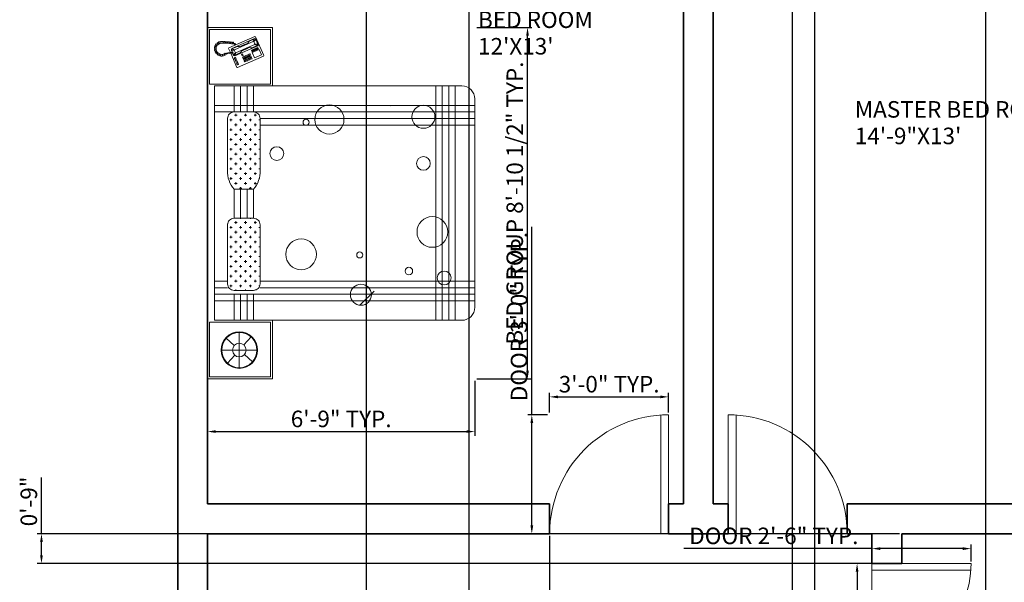
# Model space of a CAD drawing. Units: inches. Extents: x 1265 to 2734, y 1741 to 2595.
# Tile 8 of 10: x 2281 to 2579, y 2294 to 2464. Entities that reach past the tile are written whole.
import ezdxf

# ---------------------------------------------------------------- set-up
doc = ezdxf.new("R2010")
doc.units = ezdxf.units.IN
doc.header["$LTSCALE"] = 0.1
for name, color, linetype, lineweight in [('A-ANNO-DIMS', 2, 'Continuous', 18), ('A-AREA-IDEN', 7, 'Continuous', 18), ('A-DOOR', 3, 'Continuous', 18), ('A-WALL', 7, 'Continuous', 35), ('C-PROP', 7, 'Continuous', 35), ('Furniture', 8, 'Continuous', 15)]:
    doc.layers.add(name, color=color, linetype=linetype, lineweight=lineweight)
doc.styles.get("Standard").update_dxf_attribs({"font": 'arial.ttf', "height": 5})
doc.dimstyles.new('ISO-25', dxfattribs={"dimtxt": 5, "dimasz": 2.5, "dimexe": 1.25, "dimexo": 0.625, "dimtad": 1, "dimlunit": 3, "dimtxsty": 'Standard', "dimcen": 2.5, "dimadec": 0, "dimazin": 0, "dimtfac": 1, "dimtmove": 0, "dimatfit": 3, "dimfxl": 1, "dimarcsym": 0})

# ---------------------------------------------------------------- blocks, each defined once
blk = doc.blocks.new('DOOR-SWING-30IN')
for p, q in [((30, 0), (30, 30)), ((0.07, 2), (30, 2)), ((0, 0), (30, 0))]:
    blk.add_line(p, q)
blk.add_arc((30, 0), 30, 90, 180)
blk = doc.blocks.new('DOOR-SWING-36IN')
for p, q in [((33.6, 35.92), (33.6, 0)), ((36, 36), (36, 0)), ((36, 0), (0, 0))]:
    blk.add_line(p, q)
blk.add_arc((36, 0), 36, 90, 180)
blk = doc.blocks.new('BED-DOUBLE-WITH-NIGHTSTANDS')
h = blk.add_hatch()
h.set_pattern_fill('CROSS', color=256, scale=5.9055, angle=450, style=0)
h.set_pattern_definition([(90, (-724.7185, -618.2252), (1.476375, 1.476375), [0.7381875, -2.2145625]), (360, (-725.0876, -617.8561), (1.476375, -1.476375), [0.7381875, -2.2145625])])
h.paths.add_polyline_path([(13.93, 48.57), (8.02, 48.57, 0.414214), (6.06, 46.6), (6.06, 28.74, 0.414214), (8.02, 26.77), (13.93, 26.77, 0.414214), (15.9, 28.74), (15.9, 46.6, 0.414214)])
h.paths.add_polyline_path([(6.06, 62.99, 0.19223), (8.02, 57.33), (13.93, 57.33, 0.19223), (15.9, 62.99), (15.9, 78.74, 0.414214), (13.93, 80.71), (8.02, 80.71, 0.414214), (6.06, 78.74)])
for p, q in [((0, 0), (0, 106.3)), ((19.69, 106.3), (0, 106.3)), ((19.09, 105.71), (0.59, 105.71)), ((0.59, 105.71), (0.59, 89.17)), ((19.09, 105.71), (19.09, 89.17)), ((19.69, 106.3), (19.69, 88.58)), ((2.44, 101.15), (2.63, 101.34)), ((2.63, 101.34), (3.06, 101.2)), ((2.89, 101.55), (3.11, 101.7)), ((3.06, 101.2), (2.89, 101.55)), ((3.69, 101.46), (2.9, 100.92)), ((3.11, 101.7), (3.41, 101.48)), ((3.36, 101.88), (3.67, 101.95)), ((3.41, 101.48), (3.36, 101.88)), ((3.67, 101.95), (3.81, 101.64)), ((4.95, 101.56), (3.69, 101.46)), ((3.81, 101.64), (3.94, 101.98)), ((3.94, 101.98), (4.24, 102.02)), ((4.24, 102.02), (4.39, 101.64)), ((4.37, 102.03), (4.76, 102.08)), ((4.39, 101.64), (4.37, 102.03)), ((4.76, 102.08), (4.88, 101.72)), ((4.88, 101.72), (5.13, 102.07)), ((5.79, 101.48), (4.95, 101.56)), ((5.13, 102.07), (5.37, 102.03)), ((5.37, 102.03), (5.42, 101.66)), ((5.42, 101.66), (5.65, 101.97)), ((5.65, 101.97), (5.95, 101.95)), ((5.86, 101.55), (5.79, 101.48)), ((5.92, 101.48), (5.86, 101.55)), ((6.5, 101.45), (5.92, 101.48)), ((5.95, 101.95), (5.98, 101.59)), ((5.98, 101.59), (6.16, 101.92)), ((6.16, 101.92), (6.47, 101.91)), ((14.35, 103.55), (6.45, 100.09)), ((6.47, 101.91), (6.46, 101.54)), ((6.46, 101.54), (6.62, 101.9)), ((7.29, 101.35), (6.5, 101.45)), ((6.62, 101.9), (6.85, 101.89)), ((6.85, 101.89), (6.89, 101.51)), ((6.89, 101.51), (7.15, 101.84)), ((7.15, 101.84), (7.36, 101.82)), ((7.73, 101.29), (7.29, 101.35)), ((14.21, 102.94), (7.34, 99.94)), ((7.36, 101.82), (7.4, 101.48)), ((7.4, 101.48), (7.62, 101.8)), ((7.62, 101.8), (7.77, 101.81)), ((7.79, 101.48), (7.73, 101.29)), ((7.77, 101.81), (7.86, 101.7)), ((7.84, 101.37), (7.79, 101.48)), ((7.94, 101.33), (7.84, 101.37)), ((7.86, 101.7), (7.96, 101.49)), ((8.11, 101.22), (7.94, 101.33)), ((7.96, 101.49), (8.25, 101.43)), ((8.25, 101.43), (8.4, 101.32)), ((8.4, 101.32), (8.57, 101.02)), ((11.78, 101.33), (11.2, 101.08)), ((11.28, 100.91), (13.85, 102.03)), ((12.15, 101.56), (11.78, 101.33)), ((12.36, 101.86), (12.15, 101.56)), ((12.6, 102.1), (12.36, 101.86)), ((14.14, 102.78), (12.6, 102.1)), ((14.14, 102.78), (13.85, 102.03)), ((13.85, 102.03), (13.99, 102.03)), ((13.99, 102.03), (14.61, 102.64)), ((13.99, 102.03), (14.34, 101.23)), ((14.4, 102.82), (14.14, 102.78)), ((14.62, 102.78), (14.21, 102.94)), ((14.52, 103.48), (14.35, 103.55)), ((14.61, 102.64), (14.4, 102.82)), ((17.02, 97.76), (14.52, 103.48)), ((15.21, 101.26), (14.61, 102.64)), ((15.37, 101.06), (14.62, 102.78)), ((2.06, 100.15), (2.14, 100.41)), ((2.46, 100.04), (2.06, 100.15)), ((2.09, 99.7), (2.1, 99.92)), ((2.44, 99.53), (2.09, 99.7)), ((2.1, 99.92), (2.46, 100.04)), ((2.13, 99.38), (2.44, 99.53)), ((2.17, 99.14), (2.13, 99.38)), ((2.14, 100.41), (2.51, 100.41)), ((2.59, 99.17), (2.17, 99.14)), ((2.23, 100.67), (2.3, 100.88)), ((2.51, 100.41), (2.23, 100.67)), ((2.29, 98.95), (2.59, 99.17)), ((2.4, 98.76), (2.29, 98.95)), ((2.3, 100.88), (2.69, 100.86)), ((2.78, 98.76), (2.4, 98.76)), ((2.69, 100.86), (2.44, 101.15)), ((2.53, 98.47), (2.78, 98.76)), ((2.71, 98.26), (2.53, 98.47)), ((2.9, 100.92), (2.62, 100.19)), ((2.62, 100.19), (2.62, 99.39)), ((2.62, 99.39), (2.99, 98.72)), ((3.07, 98.46), (2.71, 98.26)), ((2.96, 98.08), (3.07, 98.46)), ((2.99, 98.72), (3.58, 98.25)), ((4.33, 98.05), (5.08, 98.31)), ((5.08, 98.31), (5.33, 98.48)), ((5.33, 98.48), (5.57, 98.34)), ((5.57, 98.34), (5.87, 98.48)), ((5.98, 98.32), (5.68, 98.18)), ((5.87, 98.48), (6.16, 98.57)), ((6.58, 98.42), (5.98, 98.32)), ((6.16, 98.57), (6.77, 98.66)), ((6.45, 100.09), (6.38, 99.93)), ((6.38, 99.93), (6.92, 98.7)), ((7.23, 98.53), (6.58, 98.42)), ((6.77, 98.66), (7.17, 98.75)), ((7.01, 98.5), (8.89, 94.2)), ((7.34, 99.94), (7.12, 99.5)), ((7.12, 99.5), (7.41, 98.83)), ((7.17, 98.75), (7.65, 98.91)), ((7.23, 99.41), (7.24, 99.69)), ((8.1, 99.45), (7.23, 99.41)), ((7.47, 98.85), (7.23, 99.41)), ((7.72, 98.74), (7.23, 98.53)), ((7.24, 99.69), (7.44, 99.85)), ((7.44, 99.85), (8.99, 100.52)), ((7.44, 99.85), (8.18, 99.56)), ((7.49, 98.64), (7.84, 97.84)), ((7.83, 98.04), (7.55, 98.67)), ((7.65, 98.91), (7.72, 98.74)), ((8.45, 98.65), (7.83, 98.04)), ((8.18, 99.56), (8.1, 99.45)), ((8.1, 99.45), (8.45, 98.65)), ((8.26, 101.14), (8.11, 101.22)), ((11.28, 100.91), (8.18, 99.56)), ((8.4, 100.95), (8.26, 101.14)), ((8.26, 97.68), (15.19, 100.71)), ((8.3, 97.9), (8.59, 98.64)), ((8.3, 97.9), (9.84, 98.58)), ((8.59, 98.64), (8.45, 98.65)), ((11.68, 99.99), (8.59, 98.64)), ((8.99, 100.52), (9.33, 100.53)), ((9.33, 100.53), (9.69, 100.49)), ((9.69, 100.49), (10.11, 100.6)), ((9.84, 98.58), (10.08, 98.82)), ((10.08, 98.82), (10.29, 99.11)), ((10.11, 100.6), (11.2, 101.08)), ((10.29, 99.11), (10.66, 99.34)), ((10.66, 99.34), (11.75, 99.82)), ((11.68, 99.99), (14.26, 101.12)), ((12.33, 100.07), (11.75, 99.82)), ((12.75, 100.19), (12.33, 100.07)), ((12.82, 98.31), (12.48, 98.16)), ((13.11, 100.14), (12.75, 100.19)), ((12.97, 97.97), (12.82, 98.31)), ((13.45, 100.15), (13.11, 100.14)), ((13.3, 99.4), (13.47, 99.48)), ((13.5, 98.95), (13.3, 99.4)), ((15, 100.83), (13.45, 100.15)), ((15.58, 99.65), (13.46, 98.72)), ((13.46, 98.72), (14.19, 97.06)), ((13.47, 99.48), (13.67, 99.02)), ((13.67, 99.02), (13.5, 98.95)), ((13.64, 99.55), (13.81, 99.63)), ((13.84, 99.1), (13.64, 99.55)), ((13.81, 99.63), (14.01, 99.17)), ((14.01, 99.17), (13.84, 99.1)), ((13.99, 99.7), (14.16, 99.78)), ((14.19, 99.25), (13.99, 99.7)), ((14.16, 99.78), (14.36, 99.32)), ((14.36, 99.32), (14.19, 99.25)), ((14.26, 101.12), (14.34, 101.23)), ((15, 100.83), (14.26, 101.12)), ((14.33, 99.85), (14.5, 99.93)), ((14.53, 99.4), (14.33, 99.85)), ((14.34, 101.23), (15.21, 101.26)), ((14.5, 99.93), (14.7, 99.47)), ((14.7, 99.47), (14.53, 99.4)), ((14.67, 100), (14.85, 100.08)), ((14.87, 99.55), (14.67, 100)), ((14.85, 100.08), (15.05, 99.62)), ((15.05, 99.62), (14.87, 99.55)), ((15.2, 100.99), (15, 100.83)), ((15.02, 100.16), (15.19, 100.23)), ((15.22, 99.7), (15.02, 100.16)), ((15.19, 100.71), (15.37, 101.06)), ((15.19, 100.23), (15.39, 99.77)), ((15.21, 101.26), (15.2, 100.99)), ((15.39, 99.77), (15.22, 99.7)), ((16.3, 97.99), (15.58, 99.65)), ((3.2, 97.92), (2.96, 98.08)), ((3.49, 98.1), (3.2, 97.92)), ((3.41, 97.75), (3.49, 98.1)), ((3.7, 97.67), (3.41, 97.75)), ((3.58, 98.25), (4.33, 98.05)), ((3.95, 97.97), (3.7, 97.67)), ((4.03, 97.59), (3.95, 97.97)), ((4.36, 97.56), (4.03, 97.59)), ((4.48, 97.99), (4.36, 97.56)), ((4.67, 97.64), (4.48, 97.99)), ((5, 97.75), (4.67, 97.64)), ((5.05, 98.16), (5, 97.75)), ((5.26, 97.85), (5.05, 98.16)), ((5.53, 98), (5.26, 97.85)), ((5.6, 98.18), (5.53, 98)), ((5.68, 98.18), (5.6, 98.18)), ((7.83, 98.04), (8.04, 97.86)), ((7.84, 97.84), (8.26, 97.68)), ((8.04, 97.86), (8.3, 97.9)), ((8.09, 97.13), (8.43, 97.28)), ((8.34, 96.55), (8.09, 97.13)), ((8.68, 96.7), (8.34, 96.55)), ((8.43, 97.28), (8.68, 96.7)), ((8.44, 96.33), (8.78, 96.48)), ((8.69, 95.75), (8.44, 96.33)), ((9.03, 95.9), (8.69, 95.75)), ((8.78, 96.48), (9.03, 95.9)), ((8.79, 95.52), (9.13, 95.67)), ((9.04, 94.95), (8.79, 95.52)), ((9.05, 94.14), (16.96, 97.59)), ((9.13, 95.67), (9.38, 95.1)), ((10.58, 98.29), (10.24, 98.14)), ((10.24, 98.14), (10.44, 97.68)), ((10.44, 97.68), (10.78, 97.83)), ((10.78, 97.83), (10.58, 98.29)), ((10.93, 97.48), (10.59, 97.33)), ((10.59, 97.33), (10.74, 96.99)), ((10.74, 96.99), (11.08, 97.14)), ((11.18, 96.91), (10.84, 96.76)), ((10.84, 96.76), (10.99, 96.42)), ((11.08, 97.14), (10.93, 97.48)), ((10.99, 96.42), (11.33, 96.57)), ((11.43, 96.34), (11.09, 96.19)), ((11.09, 96.19), (11.24, 95.84)), ((11.33, 96.57), (11.18, 96.91)), ((11.56, 97.76), (11.22, 97.61)), ((11.22, 97.61), (11.37, 97.26)), ((11.24, 95.84), (11.58, 95.99)), ((11.37, 97.26), (11.71, 97.42)), ((11.58, 95.99), (11.43, 96.34)), ((11.81, 97.19), (11.47, 97.04)), ((11.47, 97.04), (11.62, 96.69)), ((11.71, 97.42), (11.56, 97.76)), ((11.62, 96.69), (11.96, 96.84)), ((12.06, 96.61), (11.72, 96.46)), ((11.72, 96.46), (11.87, 96.12)), ((11.96, 96.84), (11.81, 97.19)), ((12.19, 98.03), (11.85, 97.88)), ((11.85, 97.88), (12, 97.54)), ((11.87, 96.12), (12.21, 96.27)), ((12, 97.54), (12.34, 97.69)), ((12.21, 96.27), (12.06, 96.61)), ((12.44, 97.46), (12.1, 97.31)), ((12.1, 97.31), (12.25, 96.97)), ((12.34, 97.69), (12.19, 98.03)), ((12.25, 96.97), (12.59, 97.12)), ((12.69, 96.89), (12.35, 96.74)), ((12.35, 96.74), (12.5, 96.39)), ((12.59, 97.12), (12.44, 97.46)), ((12.48, 98.16), (12.63, 97.82)), ((12.5, 96.39), (12.84, 96.55)), ((12.63, 97.82), (12.97, 97.97)), ((12.84, 96.55), (12.69, 96.89)), ((13.07, 97.74), (12.73, 97.59)), ((12.73, 97.59), (12.88, 97.24)), ((12.88, 97.24), (13.22, 97.39)), ((13.32, 97.16), (12.98, 97.01)), ((12.98, 97.01), (13.13, 96.67)), ((13.22, 97.39), (13.07, 97.74)), ((13.13, 96.67), (13.47, 96.82)), ((13.47, 96.82), (13.32, 97.16)), ((14.19, 97.06), (16.3, 97.99)), ((16.96, 97.59), (17.02, 97.76)), ((8.89, 94.2), (9.05, 94.14)), ((9.38, 95.1), (9.04, 94.95)), ((19.09, 89.17), (0.59, 89.17)), ((0.59, 89.17), (19.09, 89.17)), ((2.12, 17.72), (2.12, 88.58)), ((2.12, 88.58), (76.92, 88.58)), ((80.86, 84.65), (80.86, 21.65)), ((55.34, 82.68), (55.28, 82.62)), ((6.07, 78.97), (6.07, 62.76)), ((6.07, 46.84), (6.07, 28.51)), ((6.07, 44.57), (6.06, 44.56)), ((50.36, 26.51), (46.1, 22.26)), ((19.09, 17.13), (0.59, 17.13)), ((0.59, 0.59), (0.59, 17.13)), ((76.92, 17.72), (2.12, 17.72)), ((19.09, 0.59), (19.09, 17.13)), ((19.69, 0), (19.69, 17.72)), ((8.07, 10.1), (5.65, 12.3)), ((9.61, 8.71), (9.61, 14.05)), ((11, 10.24), (13.2, 12.67)), ((9.61, 8.71), (4.26, 8.71)), ((8.22, 7.18), (6.02, 4.75)), ((9.61, 8.71), (14.95, 8.71)), ((9.61, 8.71), (9.61, 3.36)), ((11.14, 7.32), (13.57, 5.12)), ((19.69, 0), (0, 0)), ((19.09, 0.59), (0.59, 0.59))]:
    blk.add_line(p, q)
for points in [[(8.02, 88.58), (8.02, 80.71)], [(9.99, 80.71), (9.99, 88.58), (8.02, 88.58)], [(13.93, 80.71), (13.93, 88.58), (11.96, 88.58)], [(11.96, 88.58), (11.96, 80.71)], [(2.12, 80.71), (80.86, 80.71), (80.86, 82.68), (2.12, 82.68)], [(15.9, 76.77), (80.86, 76.77), (80.86, 78.74), (15.9, 78.74)], [(8.02, 57.33), (8.02, 48.57)], [(9.99, 48.57), (9.99, 57.33)], [(11.96, 57.33), (11.96, 48.57)], [(13.93, 48.57), (13.93, 57.33)], [(2.12, 29.53), (6.06, 29.53)], [(6.06, 27.56), (2.12, 27.56)], [(15.9, 29.53), (80.86, 29.53), (80.86, 27.56), (15.9, 27.56)], [(2.12, 25.59), (80.86, 25.59), (80.86, 23.62), (2.12, 23.62)], [(8.02, 25.59), (8.02, 17.72), (9.99, 17.72), (9.99, 25.59)], [(11.96, 25.59), (11.96, 17.72), (13.93, 17.72), (13.93, 25.59)]]:
    blk.add_lwpolyline(points)
for points in [[(69.05, 88.58), (69.05, 17.72), (71.02, 17.72), (71.02, 88.58)], [(72.98, 88.58), (72.98, 17.72), (74.95, 17.72), (74.95, 88.58)]]:
    blk.add_lwpolyline(points, close=True)
for points in [[(15.9, 62.99), (15.9, 78.74, 0.414214), (13.93, 80.71), (8.02, 80.71, 0.414214), (6.06, 78.74), (6.06, 62.99, 0.19223), (8.02, 57.33), (13.93, 57.33, 0.19223)], [(15.9, 28.74), (15.9, 46.6, 0.414214), (13.93, 48.57), (8.02, 48.57, 0.414214), (6.06, 46.6), (6.06, 28.74, 0.414214), (8.02, 26.77), (13.93, 26.77, 0.414214)]]:
    blk.add_lwpolyline(points, format="xyb", close=True)
for centre, radius in [((36.86, 78.44), 4.41), ((65.32, 79.25), 3.48), ((29.81, 77.62), 0.925), ((20.97, 68.13), 2.09), ((65.3, 65.16), 2.09), ((68.02, 44.43), 4.65), ((28.31, 37.66), 4.65), ((46.05, 37.48), 0.925), ((60.91, 32.6), 1.14), ((71.58, 30.51), 2.09), ((46.4, 25.43), 3.19), ((9.61, 8.71), 5.54), ((9.61, 8.71), 5.34), ((9.61, 8.71), 2.07)]:
    blk.add_circle(centre, radius)
for centre, start, end in [((76.92, 84.65), 0, 90), ((76.92, 21.65), 270, 0)]:
    blk.add_arc(centre, 3.94, start, end)
blk = doc.blocks.new('*D16')
at = {"layer": 'A-ANNO-DIMS', "color": 0, "lineweight": -2, "transparency": 16777216}
for p, q in [((2419.09, 2461.81), (2435.66, 2461.81)), ((2434.41, 2358.01), (2434.41, 2459.31)), ((2419.09, 2355.51), (2435.66, 2355.51))]:
    blk.add_line(p, q, dxfattribs=at)
at = {"layer": 'A-ANNO-DIMS', "color": 0, "lineweight": 100, "transparency": 16777216}
for points in [[(2433.99, 2459.31), (2434.82, 2459.31), (2434.41, 2461.81)], [(2433.99, 2358.01), (2434.82, 2358.01), (2434.41, 2355.51)]]:
    blk.add_solid(points, dxfattribs=at)
at = {"layer": 'Defpoints', "color": 0, "lineweight": 100, "transparency": 16777216}
for p in [(2418.46, 2461.81), (2434.41, 2461.81), (2418.46, 2355.51)]:
    blk.add_point(p, dxfattribs=at)
at = {"layer": 'A-ANNO-DIMS', "color": 0, "transparency": 16777216, "insert": (2431.19, 2408.66), "char_height": 5, "attachment_point": 5, "rotation": 90}
blk.add_mtext('BED GROUP 8\'-10 1/2" TYP.', dxfattribs=at)
blk = doc.blocks.new('*D17')
at = {"layer": 'A-ANNO-DIMS', "color": 0, "lineweight": -2, "transparency": 16777216}
for p, q in [((2337.6, 2354.88), (2337.6, 2338.31)), ((2418.46, 2354.88), (2418.46, 2338.31)), ((2340.1, 2339.56), (2415.96, 2339.56))]:
    blk.add_line(p, q, dxfattribs=at)
at = {"layer": 'A-ANNO-DIMS', "color": 0, "lineweight": 100, "transparency": 16777216}
for points in [[(2340.1, 2339.98), (2340.1, 2339.15), (2337.6, 2339.56)], [(2415.96, 2339.98), (2415.96, 2339.15), (2418.46, 2339.56)]]:
    blk.add_solid(points, dxfattribs=at)
at = {"layer": 'Defpoints', "color": 0, "lineweight": 100, "transparency": 16777216}
for p in [(2337.6, 2355.51), (2418.46, 2355.51), (2418.46, 2339.56)]:
    blk.add_point(p, dxfattribs=at)
at = {"layer": 'A-ANNO-DIMS', "color": 0, "transparency": 16777216, "insert": (2378.03, 2342.74), "char_height": 5, "attachment_point": 5}
blk.add_mtext('6\'-9" TYP.', dxfattribs=at)
blk = doc.blocks.new('*D24')
at = {"layer": 'A-ANNO-DIMS', "color": 0, "lineweight": -2, "transparency": 16777216}
for p, q in [((2538.6, 2304.16), (2481.73, 2304.16)), ((2538.6, 2300.28), (2538.6, 2305.41)), ((2566.1, 2304.16), (2541.1, 2304.16)), ((2568.6, 2300.28), (2568.6, 2305.41))]:
    blk.add_line(p, q, dxfattribs=at)
at = {"layer": 'A-ANNO-DIMS', "color": 0, "lineweight": 100, "transparency": 16777216}
for points in [[(2541.1, 2304.57), (2541.1, 2303.74), (2538.6, 2304.16)], [(2566.1, 2304.57), (2566.1, 2303.74), (2568.6, 2304.16)]]:
    blk.add_solid(points, dxfattribs=at)
at = {"layer": 'Defpoints', "color": 0, "lineweight": 100, "transparency": 16777216}
for p in [(2538.6, 2304.16), (2538.6, 2299.66), (2568.6, 2299.66)]:
    blk.add_point(p, dxfattribs=at)
at = {"layer": 'A-ANNO-DIMS', "color": 0, "transparency": 16777216, "insert": (2508.92, 2307.37), "char_height": 5, "attachment_point": 5}
blk.add_mtext('DOOR 2\'-6" TYP.', dxfattribs=at)
blk = doc.blocks.new('*D25')
at = {"layer": 'A-ANNO-DIMS', "color": 0, "lineweight": -2, "transparency": 16777216}
for p, q in [((2537.98, 2299.66), (2532.85, 2299.66)), ((2534.1, 2297.16), (2534.1, 2272.16)), ((2537.98, 2269.66), (2532.85, 2269.66)), ((2534.1, 2269.66), (2534.1, 2235.34))]:
    blk.add_line(p, q, dxfattribs=at)
at = {"layer": 'A-ANNO-DIMS', "color": 0, "lineweight": 100, "transparency": 16777216}
for points in [[(2533.69, 2297.16), (2534.52, 2297.16), (2534.1, 2299.66)], [(2533.69, 2272.16), (2534.52, 2272.16), (2534.1, 2269.66)]]:
    blk.add_solid(points, dxfattribs=at)
at = {"layer": 'Defpoints', "color": 0, "lineweight": 100, "transparency": 16777216}
for p in [(2538.6, 2299.66), (2534.1, 2269.66), (2538.6, 2269.66)]:
    blk.add_point(p, dxfattribs=at)
at = {"layer": 'A-ANNO-DIMS', "color": 0, "transparency": 16777216, "insert": (2530.92, 2251.25), "char_height": 5, "attachment_point": 5, "rotation": 90}
blk.add_mtext('2\'-6" TYP.', dxfattribs=at)
blk = doc.blocks.new('*D26')
at = {"layer": 'A-ANNO-DIMS', "color": 0, "lineweight": -2, "transparency": 16777216}
for p, q in [((2435.7, 2344.66), (2435.7, 2401.53)), ((2440.48, 2344.66), (2434.45, 2344.66)), ((2435.7, 2311.16), (2435.7, 2342.16)), ((2440.48, 2308.66), (2434.45, 2308.66))]:
    blk.add_line(p, q, dxfattribs=at)
at = {"layer": 'A-ANNO-DIMS', "color": 0, "lineweight": 100, "transparency": 16777216}
for points in [[(2435.29, 2342.16), (2436.12, 2342.16), (2435.7, 2344.66)], [(2435.29, 2311.16), (2436.12, 2311.16), (2435.7, 2308.66)]]:
    blk.add_solid(points, dxfattribs=at)
at = {"layer": 'Defpoints', "color": 0, "lineweight": 100, "transparency": 16777216}
for p in [(2435.7, 2344.66), (2441.1, 2344.66), (2441.1, 2308.66)]:
    blk.add_point(p, dxfattribs=at)
at = {"layer": 'A-ANNO-DIMS', "color": 0, "transparency": 16777216, "insert": (2432.49, 2374.34), "char_height": 5, "attachment_point": 5, "rotation": 90}
blk.add_mtext('DOOR 3\'-0" TYP.', dxfattribs=at)
blk = doc.blocks.new('*D27')
at = {"layer": 'A-ANNO-DIMS', "color": 0, "lineweight": -2, "transparency": 16777216}
for p, q in [((2441.1, 2345.28), (2441.1, 2351.31)), ((2477.1, 2345.28), (2477.1, 2351.31)), ((2443.6, 2350.06), (2474.6, 2350.06))]:
    blk.add_line(p, q, dxfattribs=at)
at = {"layer": 'A-ANNO-DIMS', "color": 0, "lineweight": 100, "transparency": 16777216}
for points in [[(2443.6, 2350.47), (2443.6, 2349.64), (2441.1, 2350.06)], [(2474.6, 2350.47), (2474.6, 2349.64), (2477.1, 2350.06)]]:
    blk.add_solid(points, dxfattribs=at)
at = {"layer": 'Defpoints', "color": 0, "lineweight": 100, "transparency": 16777216}
for p in [(2477.1, 2350.06), (2441.1, 2344.66), (2477.1, 2344.66)]:
    blk.add_point(p, dxfattribs=at)
at = {"layer": 'A-ANNO-DIMS', "color": 0, "transparency": 16777216, "insert": (2459.1, 2353.24), "char_height": 5, "attachment_point": 5}
blk.add_mtext('3\'-0" TYP.', dxfattribs=at)
blk = doc.blocks.new('*D42')
at = {"layer": 'A-ANNO-DIMS', "color": 0, "lineweight": -2, "transparency": 16777216}
for p, q in [((2328.6, 1822.68), (2328.6, 2585.16)), ((2331.1, 2583.91), (2518.82, 2583.91)), ((2521.32, 1822.68), (2521.32, 2585.16))]:
    blk.add_line(p, q, dxfattribs=at)
at = {"layer": 'A-ANNO-DIMS', "color": 0, "lineweight": 100, "transparency": 16777216}
for points in [[(2331.1, 2584.32), (2331.1, 2583.49), (2328.6, 2583.91)], [(2518.82, 2584.32), (2518.82, 2583.49), (2521.32, 2583.91)]]:
    blk.add_solid(points, dxfattribs=at)
at = {"layer": 'Defpoints', "color": 0, "lineweight": 100, "transparency": 16777216}
for p in [(2521.32, 2583.91), (2328.6, 1822.06), (2521.32, 1822.06)]:
    blk.add_point(p, dxfattribs=at)
at = {"layer": 'A-ANNO-DIMS', "color": 0, "transparency": 16777216, "insert": (2424.96, 2587.12), "char_height": 5, "attachment_point": 5}
blk.add_mtext('16\'-0 1/2"', dxfattribs=at)
blk = doc.blocks.new('*D43')
at = {"layer": 'A-ANNO-DIMS', "color": 0, "lineweight": -2, "transparency": 16777216}
for p, q in [((2337.6, 2308.03), (2337.6, 1744.16)), ((2441.1, 2308.03), (2441.1, 1744.16)), ((2340.1, 1745.41), (2438.6, 1745.41))]:
    blk.add_line(p, q, dxfattribs=at)
at = {"layer": 'A-ANNO-DIMS', "color": 0, "lineweight": 100, "transparency": 16777216}
for points in [[(2340.1, 1745.82), (2340.1, 1744.99), (2337.6, 1745.41)], [(2438.6, 1745.82), (2438.6, 1744.99), (2441.1, 1745.41)]]:
    blk.add_solid(points, dxfattribs=at)
at = {"layer": 'Defpoints', "color": 0, "lineweight": 100, "transparency": 16777216}
for p in [(2337.6, 2308.66), (2441.1, 2308.66), (2441.1, 1745.41)]:
    blk.add_point(p, dxfattribs=at)
at = {"layer": 'A-ANNO-DIMS', "color": 0, "transparency": 16777216, "insert": (2389.35, 1748.62), "char_height": 5, "attachment_point": 5}
blk.add_mtext('8\'-7 1/2"', dxfattribs=at)
blk = doc.blocks.new('*D45')
at = {"layer": 'A-ANNO-DIMS', "color": 0, "lineweight": -2, "transparency": 16777216}
for p, q in [((2385.6, 2477.53), (2385.6, 1744.16)), ((2416.67, 2477.91), (2416.67, 1744.16)), ((2388.1, 1745.41), (2414.17, 1745.41))]:
    blk.add_line(p, q, dxfattribs=at)
at = {"layer": 'A-ANNO-DIMS', "color": 0, "lineweight": 100, "transparency": 16777216}
for points in [[(2388.1, 1745.82), (2388.1, 1744.99), (2385.6, 1745.41)], [(2414.17, 1745.82), (2414.17, 1744.99), (2416.67, 1745.41)]]:
    blk.add_solid(points, dxfattribs=at)
at = {"layer": 'Defpoints', "color": 0, "lineweight": 100, "transparency": 16777216}
for p in [(2416.67, 2478.54), (2385.6, 2478.16), (2416.67, 1745.41)]:
    blk.add_point(p, dxfattribs=at)
at = {"layer": 'A-ANNO-DIMS', "color": 0, "transparency": 16777216, "insert": (2401.14, 1748.54), "char_height": 5, "attachment_point": 5}
blk.add_mtext('2\'-7"', dxfattribs=at)
blk = doc.blocks.new('*D47')
at = {"layer": 'A-ANNO-DIMS', "color": 0, "lineweight": -2, "transparency": 16777216}
for p, q in [((2514.6, 1992.78), (2514.6, 2585.16)), ((2517.1, 2583.91), (2570.6, 2583.91)), ((2573.1, 1992.78), (2573.1, 2585.16))]:
    blk.add_line(p, q, dxfattribs=at)
at = {"layer": 'A-ANNO-DIMS', "color": 0, "lineweight": 100, "transparency": 16777216}
for points in [[(2517.1, 2584.32), (2517.1, 2583.49), (2514.6, 2583.91)], [(2570.6, 2584.32), (2570.6, 2583.49), (2573.1, 2583.91)]]:
    blk.add_solid(points, dxfattribs=at)
at = {"layer": 'Defpoints', "color": 0, "lineweight": 100, "transparency": 16777216}
for p in [(2573.1, 2583.91), (2514.6, 1992.16), (2573.1, 1992.16)]:
    blk.add_point(p, dxfattribs=at)
at = {"layer": 'A-ANNO-DIMS', "color": 0, "transparency": 16777216, "insert": (2543.85, 2587.12), "char_height": 5, "attachment_point": 5}
blk.add_mtext('4\'-10 1/2"', dxfattribs=at)
blk = doc.blocks.new('*D49')
at = {"layer": 'A-ANNO-DIMS', "color": 0, "lineweight": -2, "transparency": 16777216}
for p, q in [((2287.35, 2308.66), (2287.35, 2325.7)), ((2546.98, 2308.66), (2286.1, 2308.66)), ((2287.35, 2302.16), (2287.35, 2306.16)), ((2546.98, 2299.66), (2286.1, 2299.66))]:
    blk.add_line(p, q, dxfattribs=at)
at = {"layer": 'A-ANNO-DIMS', "color": 0, "lineweight": 100, "transparency": 16777216}
for points in [[(2286.94, 2306.16), (2287.77, 2306.16), (2287.35, 2308.66)], [(2286.94, 2302.16), (2287.77, 2302.16), (2287.35, 2299.66)]]:
    blk.add_solid(points, dxfattribs=at)
at = {"layer": 'Defpoints', "color": 0, "lineweight": 100, "transparency": 16777216}
for p in [(2287.35, 2308.66), (2547.6, 2308.66), (2547.6, 2299.66)]:
    blk.add_point(p, dxfattribs=at)
at = {"layer": 'A-ANNO-DIMS', "color": 0, "transparency": 16777216, "insert": (2284.17, 2318.43), "char_height": 5, "attachment_point": 5, "rotation": 90}
blk.add_mtext('0\'-9"', dxfattribs=at)

msp = doc.modelspace()

# ---------------------------------------------------------------- linework, layer by layer
at = {"layer": 'A-WALL'}
for p, q in [((2481.602, 2317.657), (2481.602, 2482.657)), ((2490.602, 2317.657), (2490.602, 2482.657)), ((2337.602, 2317.657), (2337.602, 2473.657)), ((2337.602, 2317.657), (2441.102, 2317.657)), ((2441.102, 2317.657), (2441.102, 2308.657)), ((2477.102, 2317.657), (2477.102, 2308.657)), ((2477.102, 2317.657), (2481.602, 2317.657)), ((2490.602, 2317.657), (2495.102, 2317.657)), ((2495.102, 2317.657), (2495.102, 2308.657)), ((2531.102, 2317.657), (2531.102, 2308.657)), ((2531.102, 2317.657), (2679.602, 2317.657)), ((2337.602, 2308.657), (2441.102, 2308.657)), ((2337.602, 2140.657), (2337.602, 2308.657)), ((2477.102, 2308.657), (2495.102, 2308.657)), ((2531.102, 2308.657), (2538.602, 2308.657)), ((2538.602, 2308.657), (2538.602, 2299.657)), ((2547.602, 2308.657), (2547.602, 2299.657)), ((2547.602, 2308.657), (2547.602, 2299.657)), ((2547.602, 2308.657), (2679.602, 2308.657)), ((2538.602, 2299.657), (2547.602, 2299.657))]:
    msp.add_line(p, q, dxfattribs=at)
at = {"layer": 'C-PROP'}
msp.add_line((2328.602, 1786.657), (2328.602, 2542.657), dxfattribs=at)

# ---------------------------------------------------------------- block references
at = {"layer": 'A-DOOR'}
msp.add_blockref('DOOR-SWING-36IN', (2441.102, 2308.657), dxfattribs=at)
at = {"layer": 'A-DOOR', "extrusion": (0, 0, -1), "zscale": -1}
msp.add_blockref('DOOR-SWING-36IN', (-2531.103, 2308.657), dxfattribs=at)
at = {"layer": 'A-DOOR', "rotation": 180}
msp.add_blockref('DOOR-SWING-30IN', (2568.603, 2299.656), dxfattribs=at)
at = {"layer": 'Furniture'}
msp.add_blockref('BED-DOUBLE-WITH-NIGHTSTANDS', (2337.602, 2355.507), dxfattribs=at)

# ---------------------------------------------------------------- texts
at = {"layer": 'A-AREA-IDEN'}
for s, p in [('BED ROOM', (2419.434, 2461.629)), ("12'X13'", (2419.434, 2453.597)), ('MASTER BED ROOM', (2533.419, 2434.508)), ('14\'-9"X13\'', (2533.419, 2426.476))]:
    msp.add_text(s, height=5, dxfattribs=at).set_placement(p)

# ---------------------------------------------------------------- dimensions: what is measured, and where the dimension line sits
at = {"layer": 'A-ANNO-DIMS'}
for base, p1, p2, picture, middle in [((2521.319, 2583.907), (2328.602, 1822.059), (2521.319, 1822.059), '*D42', (2424.961, 2587.117)), ((2573.102, 2583.907), (2514.602, 1992.157), (2573.102, 1992.157), '*D47', (2543.852, 2587.117)), ((2416.673, 1745.407), (2385.602, 2478.157), (2416.673, 2478.538), '*D45', (2401.138, 1748.542)), ((2441.102, 1745.407), (2337.602, 2308.657), (2441.102, 2308.657), '*D43', (2389.352, 1748.617))]:
    dim = msp.add_linear_dim(base=base, p1=p1, p2=p2, dimstyle='ISO-25', override={"dimdec": 1, "dimlfac": 1, "dimrnd": 0, "dimzin": 1, "dimdsep": 46, "dimlunit": 4, "dimfrac": 2}, dxfattribs=at)
    dim.commit()
    dim.dimension.update_dxf_attribs({"geometry": picture, "text_midpoint": middle})
for base, p1, p2, angle, text, picture, middle in [((2434.405, 2461.806), (2418.461, 2355.507), (2418.461, 2461.806), 90, 'BED GROUP <> TYP.', '*D16', (2431.193, 2408.657)), ((2435.702, 2344.657), (2441.102, 2308.657), (2441.102, 2344.657), 90, 'DOOR <> TYP.', '*D26', (2432.489, 2374.344)), ((2538.602, 2304.157), (2568.602, 2299.657), (2538.602, 2299.657), 180, 'DOOR <> TYP.', '*D24', (2508.915, 2307.369)), ((2534.102, 2269.657), (2538.602, 2299.657), (2538.602, 2269.657), 270, '<> TYP.', '*D25', (2530.925, 2251.25))]:
    dim = msp.add_linear_dim(base=base, p1=p1, p2=p2, angle=angle, text=text, dimstyle='ISO-25', override={"dimdec": 1, "dimlfac": 1, "dimrnd": 0, "dimzin": 1, "dimdsep": 46, "dimlunit": 4, "dimfrac": 2}, dxfattribs=at)
    dim.commit()
    dim.dimension.update_dxf_attribs({"geometry": picture, "text_midpoint": middle})
for base, p1, p2, picture, middle in [((2477.102, 2350.057), (2441.102, 2344.657), (2477.102, 2344.657), '*D27', (2459.102, 2353.236)), ((2418.461, 2339.562), (2337.602, 2355.507), (2418.461, 2355.507), '*D17', (2378.032, 2342.74))]:
    dim = msp.add_linear_dim(base=base, p1=p1, p2=p2, text='<> TYP.', dimstyle='ISO-25', override={"dimdec": 1, "dimlfac": 1, "dimrnd": 0, "dimzin": 1, "dimdsep": 46, "dimlunit": 4, "dimfrac": 2}, dxfattribs=at)
    dim.commit()
    dim.dimension.update_dxf_attribs({"geometry": picture, "text_midpoint": middle})
dim = msp.add_linear_dim(base=(2287.352, 2308.657), p1=(2547.602, 2299.657), p2=(2547.602, 2308.657), angle=90, dimstyle='ISO-25', override={"dimdec": 1, "dimlfac": 1, "dimrnd": 0, "dimzin": 1, "dimdsep": 46, "dimlunit": 4, "dimfrac": 2}, dxfattribs=at)
dim.commit()
dim.dimension.update_dxf_attribs({"geometry": '*D49', "text_midpoint": (2284.175, 2318.427)})

doc.saveas('drawing.dxf')
